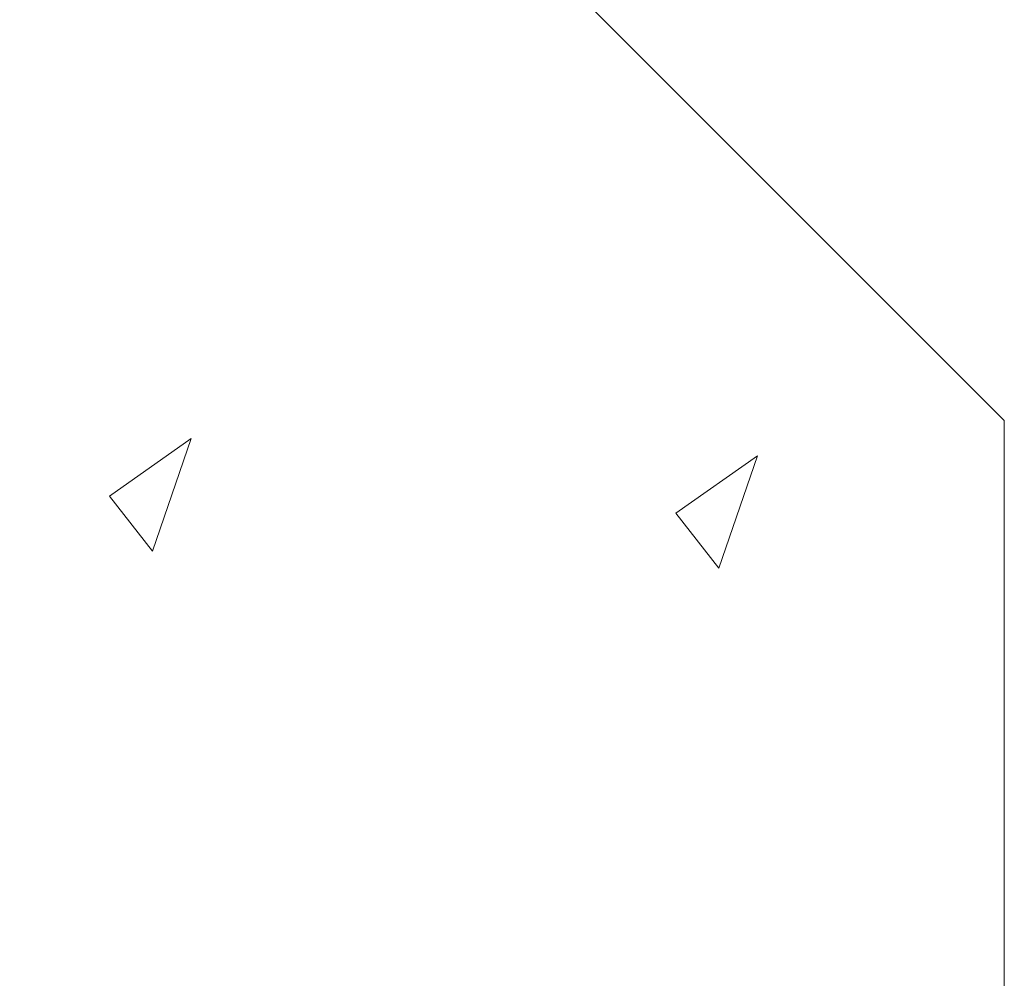
# Model space of a CAD drawing. Units: inches. Extents: x 459864 to 460310, y 324185 to 324787.
# Tile 12 of 112: x 460072.714 to 460075.876, y 324235.812 to 324238.89. Entities that reach past the tile are written whole.
import ezdxf

# ---------------------------------------------------------------- set-up
doc = ezdxf.new("R2010")
doc.units = ezdxf.units.IN
doc.layers.add('L-HRDS', color=9, linetype='Continuous', lineweight=18)

# ---------------------------------------------------------------- blocks, each defined once
blk = doc.blocks.new('Stepping Stone - hexagonal')
for p, q in [((9.0601, 4.2016), (3.1951, 10.0666)), ((9.0601, -4.0924), (9.0601, 4.2016)), ((4.7091, 4.1046), (4.2721, 3.7956)), ((4.5021, 3.5016), (4.7091, 4.1046)), ((7.7401, 4.0126), (7.3031, 3.7046)), ((7.5321, 3.4106), (7.7401, 4.0126)), ((4.2721, 3.7956), (4.5021, 3.5016)), ((7.3031, 3.7046), (7.5321, 3.4106))]:
    blk.add_line(p, q)

msp = doc.modelspace()

# ---------------------------------------------------------------- block references
at = {"layer": 'L-HRDS', "xscale": 0.6, "yscale": 0.6}
msp.add_blockref('Stepping Stone - hexagonal', (460070.4397, 324235.0823), dxfattribs=at)

doc.saveas('drawing.dxf')
